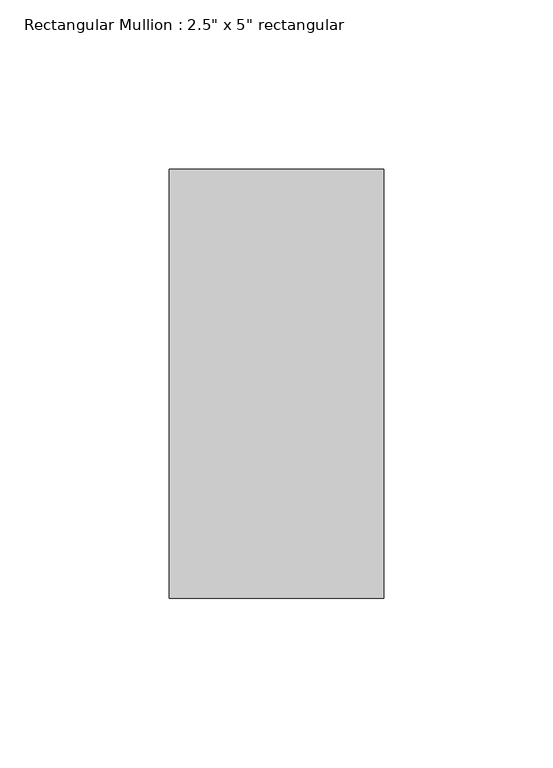
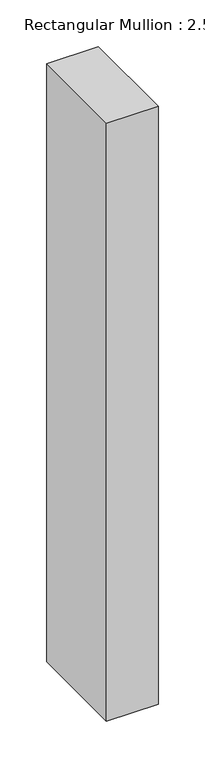
"""IFC4 building model written with IfcOpenShell, lengths in millimetres: member geometry."""

from ifc_helpers import new_model, si_unit, frame, origin, place, context, project, spatial, polyline, outline, extrude, source, transform, mapped, element, save


def member_a37bde81(model_context):
    return source(origin(), model_context, "Body", "SweptSolid", [
        extrude(outline(polyline([(0.0, 63.5), (0.0, -63.5), (-63.5, -63.5), (-63.5, 63.5), (0.0, 63.5)])), frame((0.0, 0.0, -778.426051), z_axis=(0.0, 0.0, 1.0), x_axis=(1.0, 0.0, 0.0)), (0.0, 0.0, 1.0), 778.426051),
    ])


if __name__ == "__main__":
    model = new_model("IFC4")
    model_context = context("Model", 3, world=origin())
    ifc_project = project(units=[si_unit("LENGTHUNIT", "METRE", prefix="MILLI")], contexts=[model_context])
    site = spatial("IfcSite", under=ifc_project)
    building = spatial("IfcBuilding", under=site)
    placement = place(None, origin())
    member_shape = member_a37bde81(model_context)
    element("IfcMember", 1, ObjectType="Rectangular Mullion : 2.5\" x 5\" rectangular", at=placement, inside=building, context=model_context, shape_type="MappedRepresentation", body=[
        mapped(member_shape, transform((0.0, 0.0, 0.0), x_axis=(1.0, 0.0, 0.0), y_axis=(0.0, 1.0, 0.0), z_axis=(0.0, 0.0, 1.0))),
    ])
    save(model, "model.ifc")

# Revit data of these elements
# Type "Rectangular Mullion : 2.5\" x 5\" rectangular"
#   built-in parameter 1007304 = 0.416667 (stored number, unit not read)
#   built-in parameter 1007301 = 0.104167 (stored number, unit not read)
#   built-in parameter 1007300 = 0.104167 (stored number, unit not read)
# Element 1 (IfcMember, "Rectangular Mullion : 2.5\" x 5\" rectangular")
#   Materials on its faces: "Aluminum"
# Materials
#   "Aluminum": class "Metal", colour RGB 247 247 247, transparency 0, Description = "Aluminum 6061", Cost = 0
